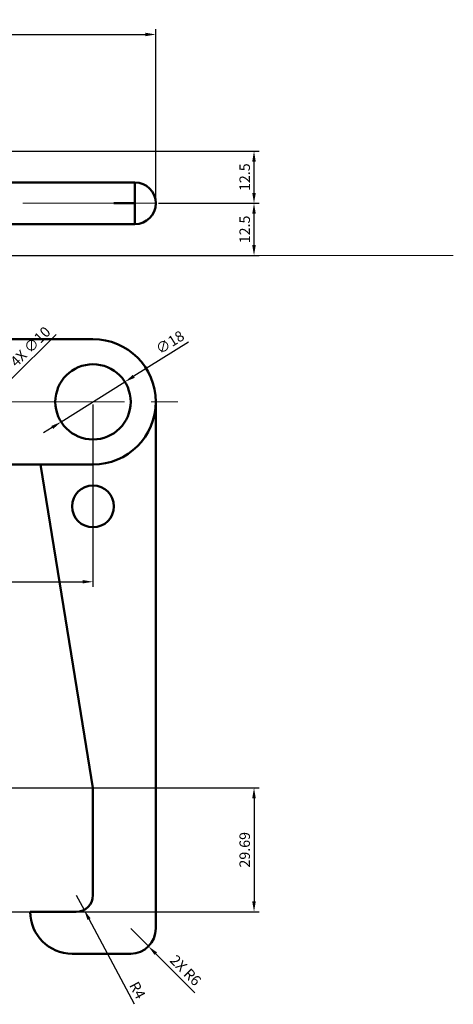
# Model space of a CAD drawing. Units: millimetres. Extents: x 5897 to 6166, y 4290 to 4529.
# Tile 2 of 2: x 6062 to 6166, y 4292 to 4528. Entities that reach past the tile are written whole.
import ezdxf

# ---------------------------------------------------------------- set-up
doc = ezdxf.new("R2010")
doc.units = ezdxf.units.MM
doc.linetypes.add('CENTER', pattern=[50.8, 31.75, -6.35, 6.35, -6.35])
for name, color, linetype, lineweight in [('M-CNTR', 1, 'CENTER', 18), ('M-CONS', 8, 'Continuous', 13), ('M-DIMS', 2, 'Continuous', 25), ('M-OUTL', 7, 'Continuous', 50)]:
    doc.layers.add(name, color=color, linetype=linetype, lineweight=lineweight)
doc.styles.get("Standard").update_dxf_attribs({"font": 'arial.ttf'})
doc.dimstyles.new('ISO-25', dxfattribs={"dimtxt": 2.5, "dimasz": 2.5, "dimexe": 1.25, "dimexo": 0.625, "dimtad": 1, "dimtxsty": 'Standard', "dimcen": 2.5, "dimadec": 0, "dimazin": 0, "dimtfac": 1, "dimtmove": 0, "dimatfit": 3, "dimfxl": 1, "dimarcsym": 0})

# ---------------------------------------------------------------- blocks, each defined once
blk = doc.blocks.new('*D9')
at = {"layer": 'Defpoints', "color": 0, "transparency": 16777216}
for p in [(5929.69, 4436.5), (6079.69, 4436.5), (6079.69, 4393.47)]:
    blk.add_point(p, dxfattribs=at)
at = {"layer": 'M-DIMS', "color": 0, "lineweight": -2, "transparency": 16777216}
for p, q in [((5929.69, 4435.88), (5929.69, 4392.22)), ((6079.69, 4435.88), (6079.69, 4392.22)), ((5932.19, 4393.47), (6077.19, 4393.47))]:
    blk.add_line(p, q, dxfattribs=at)
at = {"layer": 'M-DIMS', "color": 0, "transparency": 16777216}
for points in [[(5932.19, 4393.89), (5932.19, 4393.06), (5929.69, 4393.47)], [(6077.19, 4393.89), (6077.19, 4393.06), (6079.69, 4393.47)]]:
    blk.add_solid(points, dxfattribs=at)
at = {"layer": 'M-DIMS', "color": 0, "transparency": 16777216, "insert": (6004.69, 4395.37), "char_height": 2.5, "attachment_point": 5}
blk.add_mtext('150', dxfattribs=at)
blk = doc.blocks.new('*D10')
at = {"layer": 'Defpoints', "color": 0, "transparency": 16777216}
for p in [(6094.69, 4524.39), (5914.69, 4484), (6094.69, 4484)]:
    blk.add_point(p, dxfattribs=at)
at = {"layer": 'M-DIMS', "color": 0, "lineweight": -2, "transparency": 16777216}
for p, q in [((5914.69, 4484.63), (5914.69, 4525.64)), ((6094.69, 4484.63), (6094.69, 4525.64)), ((5917.19, 4524.39), (6092.19, 4524.39))]:
    blk.add_line(p, q, dxfattribs=at)
at = {"layer": 'M-DIMS', "color": 0, "transparency": 16777216}
for points in [[(5917.19, 4524.81), (5917.19, 4523.97), (5914.69, 4524.39)], [(6092.19, 4524.81), (6092.19, 4523.97), (6094.69, 4524.39)]]:
    blk.add_solid(points, dxfattribs=at)
at = {"layer": 'M-DIMS', "color": 0, "transparency": 16777216, "insert": (6004.69, 4526.29), "char_height": 2.5, "attachment_point": 5}
blk.add_mtext('180', dxfattribs=at)
blk = doc.blocks.new('*D14')
at = {"layer": 'Defpoints', "color": 0, "transparency": 16777216}
for p in [(6075.69, 4318.5), (6077.57, 4314.97)]:
    blk.add_point(p, dxfattribs=at)
at = {"layer": 'M-DIMS', "color": 0, "lineweight": -2, "transparency": 16777216}
for p, q in [((6075.69, 4318.5), (6077.57, 4314.97)), ((6089.62, 4292.39), (6078.75, 4312.77))]:
    blk.add_line(p, q, dxfattribs=at)
at = {"layer": 'M-DIMS', "color": 0, "transparency": 16777216}
blk.add_solid([(6079.11, 4312.96), (6078.38, 4312.57), (6077.57, 4314.97)], dxfattribs=at)
at = {"layer": 'M-DIMS', "color": 0, "transparency": 16777216, "insert": (6090.03, 4295.6), "char_height": 2.5, "attachment_point": 5, "rotation": 298.0738}
blk.add_mtext('R4', dxfattribs=at)
blk = doc.blocks.new('*D15')
at = {"layer": 'Defpoints', "color": 0, "transparency": 16777216}
for p in [(6087.31, 4441.29), (6072.07, 4431.72)]:
    blk.add_point(p, dxfattribs=at)
at = {"layer": 'M-DIMS', "color": 0, "lineweight": -2, "transparency": 16777216}
for p, q in [((6102.5, 4450.82), (6089.43, 4442.62)), ((6072.07, 4431.72), (6087.31, 4441.29)), ((6069.95, 4430.39), (6067.83, 4429.06))]:
    blk.add_line(p, q, dxfattribs=at)
at = {"layer": 'M-DIMS', "color": 0, "transparency": 16777216}
for points in [[(6089.21, 4442.97), (6089.65, 4442.26), (6087.31, 4441.29)], [(6069.73, 4430.74), (6070.17, 4430.03), (6072.07, 4431.72)]]:
    blk.add_solid(points, dxfattribs=at)
at = {"layer": 'M-DIMS', "color": 0, "transparency": 16777216, "insert": (6098.25, 4450.48), "char_height": 2.5, "attachment_point": 5, "rotation": 32.1239}
blk.add_mtext('∅18', dxfattribs=at)
blk = doc.blocks.new('*D20')
at = {"layer": 'Defpoints', "color": 0, "transparency": 16777216}
for p in [(6017.19, 4496.5), (6118.15, 4496.5), (6094.69, 4484)]:
    blk.add_point(p, dxfattribs=at)
at = {"layer": 'M-DIMS', "color": 0, "lineweight": -2, "transparency": 16777216}
for p, q in [((6017.81, 4496.5), (6119.4, 4496.5)), ((6118.15, 4486.5), (6118.15, 4494)), ((6095.31, 4484), (6119.4, 4484))]:
    blk.add_line(p, q, dxfattribs=at)
at = {"layer": 'M-DIMS', "color": 0, "transparency": 16777216}
for points in [[(6117.73, 4494), (6118.57, 4494), (6118.15, 4496.5)], [(6117.73, 4486.5), (6118.57, 4486.5), (6118.15, 4484)]]:
    blk.add_solid(points, dxfattribs=at)
at = {"layer": 'M-DIMS', "color": 0, "transparency": 16777216, "insert": (6116.25, 4490.25), "char_height": 2.5, "attachment_point": 5, "rotation": 90}
blk.add_mtext('12.5', dxfattribs=at)
blk = doc.blocks.new('*D21')
at = {"layer": 'Defpoints', "color": 0, "transparency": 16777216}
for p in [(6094.69, 4484), (6118.15, 4484), (6017.19, 4471.5)]:
    blk.add_point(p, dxfattribs=at)
at = {"layer": 'M-DIMS', "color": 0, "lineweight": -2, "transparency": 16777216}
for p, q in [((6095.31, 4484), (6119.4, 4484)), ((6118.15, 4474), (6118.15, 4481.5)), ((6017.81, 4471.5), (6119.4, 4471.5))]:
    blk.add_line(p, q, dxfattribs=at)
at = {"layer": 'M-DIMS', "color": 0, "transparency": 16777216}
for points in [[(6117.73, 4481.5), (6118.57, 4481.5), (6118.15, 4484)], [(6117.73, 4474), (6118.57, 4474), (6118.15, 4471.5)]]:
    blk.add_solid(points, dxfattribs=at)
at = {"layer": 'M-DIMS', "color": 0, "transparency": 16777216, "insert": (6116.25, 4477.75), "char_height": 2.5, "attachment_point": 5, "rotation": 90}
blk.add_mtext('12.5', dxfattribs=at)
blk = doc.blocks.new('*D25')
at = {"layer": 'Defpoints', "color": 0, "transparency": 16777216}
for p in [(5929.69, 4344.19), (5944.69, 4314.5), (6118.15, 4314.5)]:
    blk.add_point(p, dxfattribs=at)
at = {"layer": 'M-DIMS', "color": 0, "lineweight": -2, "transparency": 16777216}
for p, q in [((5930.31, 4344.19), (6119.4, 4344.19)), ((6118.15, 4341.69), (6118.15, 4317)), ((5945.31, 4314.5), (6119.4, 4314.5))]:
    blk.add_line(p, q, dxfattribs=at)
at = {"layer": 'M-DIMS', "color": 0, "transparency": 16777216}
for points in [[(6117.73, 4341.69), (6118.57, 4341.69), (6118.15, 4344.19)], [(6117.73, 4317), (6118.57, 4317), (6118.15, 4314.5)]]:
    blk.add_solid(points, dxfattribs=at)
at = {"layer": 'M-DIMS', "color": 0, "transparency": 16777216, "insert": (6116.25, 4329.35), "char_height": 2.5, "attachment_point": 5, "rotation": 90}
blk.add_mtext('29.69', dxfattribs=at)
blk = doc.blocks.new('*D35')
at = {"layer": 'Defpoints', "color": 0, "transparency": 16777216}
for p in [(6088.69, 4310.5), (6092.93, 4306.26)]:
    blk.add_point(p, dxfattribs=at)
at = {"layer": 'M-DIMS', "color": 0, "lineweight": -2, "transparency": 16777216}
for p, q in [((6088.69, 4310.5), (6092.93, 4306.26)), ((6104.03, 4295.16), (6094.7, 4304.49))]:
    blk.add_line(p, q, dxfattribs=at)
at = {"layer": 'M-DIMS', "color": 0, "transparency": 16777216}
blk.add_solid([(6094.99, 4304.79), (6094.4, 4304.2), (6092.93, 4306.26)], dxfattribs=at)
at = {"layer": 'M-DIMS', "color": 0, "transparency": 16777216, "insert": (6101.59, 4300.29), "char_height": 2.5, "attachment_point": 5, "rotation": 314.9957}
blk.add_mtext('2X R6', dxfattribs=at)
blk = doc.blocks.new('*D36')
at = {"layer": 'Defpoints', "color": 0, "transparency": 16777216}
for p in [(6058.23, 4440.03), (6051.14, 4432.97)]:
    blk.add_point(p, dxfattribs=at)
at = {"layer": 'M-DIMS', "color": 0, "lineweight": -2, "transparency": 16777216}
for p, q in [((6070.9, 4452.65), (6060, 4441.79)), ((6051.14, 4432.97), (6058.23, 4440.03)), ((6049.37, 4431.21), (6047.6, 4429.45))]:
    blk.add_line(p, q, dxfattribs=at)
at = {"layer": 'M-DIMS', "color": 0, "transparency": 16777216}
for points in [[(6059.71, 4442.09), (6060.3, 4441.5), (6058.23, 4440.03)], [(6049.08, 4431.5), (6049.67, 4430.91), (6051.14, 4432.97)]]:
    blk.add_solid(points, dxfattribs=at)
at = {"layer": 'M-DIMS', "color": 0, "transparency": 16777216, "insert": (6064.95, 4449.5), "char_height": 2.5, "attachment_point": 5, "rotation": 44.8833}
blk.add_mtext('4X ∅10', dxfattribs=at)

msp = doc.modelspace()

# ---------------------------------------------------------------- linework, layer by layer
at = {"layer": 'M-CNTR'}
for p, q in [((6094.688, 4484.002), (6004.688, 4484.002)), ((6004.688, 4436.502), (6105.301, 4436.502))]:
    msp.add_line(p, q, dxfattribs=at)
at = {"layer": 'M-CONS'}
for p, q in [((6165.744, 4471.502), (5997.188, 4471.502)), ((6004.688, 4471.502), (6165.744, 4471.502))]:
    msp.add_line(p, q, dxfattribs=at)
at = {"layer": 'M-OUTL'}
for p, q in [((6019.688, 4489.002), (6089.688, 4489.002)), ((6089.688, 4479.002), (6089.688, 4489.002)), ((6089.688, 4484.002), (6084.688, 4484.002)), ((6089.688, 4484.002), (6089.688, 4479.002)), ((6089.688, 4479.002), (6019.688, 4479.002)), ((6014.688, 4451.502), (6079.688, 4451.502)), ((6094.688, 4436.502), (6094.688, 4310.502)), ((6004.688, 4421.502), (6079.688, 4421.502)), ((6067.125, 4421.502), (6077.688, 4356.502)), ((6077.688, 4356.502), (6079.688, 4344.194)), ((6079.688, 4325.616), (6079.688, 4344.194)), ((6079.688, 4325.616), (6079.688, 4318.502)), ((6064.688, 4314.502), (6064.688, 4314.502)), ((6064.688, 4314.502), (6075.688, 4314.502)), ((6088.688, 4304.502), (6074.688, 4304.502)), ((6074.688, 4304.502), (6088.688, 4304.502)), ((6088.688, 4304.502), (6084.688, 4304.502))]:
    msp.add_line(p, q, dxfattribs=at)
for centre, radius in [((6079.688, 4436.502), 9), ((6079.688, 4411.502), 5)]:
    msp.add_circle(centre, radius, dxfattribs=at)
for centre, radius, start, end in [((6089.688, 4484.002), 5, 270, 90), ((6079.688, 4436.502), 15, 270, 90), ((6075.688, 4318.502), 4, 270, 360), ((6074.688, 4314.502), 10, 180, 270), ((6088.688, 4310.502), 6, 270, 0)]:
    msp.add_arc(centre, radius, start, end, dxfattribs=at)

# ---------------------------------------------------------------- dimensions: what is measured, and where the dimension line sits
at = {"layer": 'M-DIMS'}
for base, p1, p2, picture, middle in [((6094.688, 4524.388), (5914.688, 4484.002), (6094.688, 4484.002), '*D10', (6004.688, 4526.29)), ((6079.688, 4393.473), (5929.688, 4436.502), (6079.688, 4436.502), '*D9', (6004.688, 4395.374))]:
    dim = msp.add_linear_dim(base=base, p1=p1, p2=p2, dimstyle='ISO-25', override={"dimclrd": 0, "dimclre": 0, "dimclrt": 0}, dxfattribs=at)
    dim.commit()
    dim.dimension.update_dxf_attribs({"geometry": picture, "text_midpoint": middle})
for base, p1, p2, override, picture, middle in [((6118.151, 4496.502), (6094.688, 4484.002), (6017.188, 4496.502), {"dimdec": 1, "dimlfac": 1, "dimrnd": 0, "dimzin": 0, "dimdsep": 46, "dimlunit": 2}, '*D20', (6116.25, 4490.252)), ((6118.151, 4484.002), (6017.188, 4471.502), (6094.688, 4484.002), {"dimdec": 1, "dimlfac": 1, "dimrnd": 0, "dimzin": 0, "dimdsep": 46, "dimlunit": 2}, '*D21', (6116.25, 4477.752)), ((6118.151, 4314.502), (5929.688, 4344.194), (5944.688, 4314.502), {"dimdec": 2, "dimlfac": 1, "dimrnd": 0, "dimzin": 0, "dimdsep": 46, "dimlunit": 2}, '*D25', (6116.25, 4329.348))]:
    dim = msp.add_linear_dim(base=base, p1=p1, p2=p2, angle=90, dimstyle='ISO-25', override=override, dxfattribs=at)
    dim.commit()
    dim.dimension.update_dxf_attribs({"geometry": picture, "text_midpoint": middle})
dim = msp.add_diameter_dim_2p(p1=(6051.145, 4432.974), p2=(6058.23, 4440.03), text='4X <>', dimstyle='ISO-25', override={"dimdec": 0, "dimlfac": 1, "dimrnd": 0, "dimzin": 0, "dimdsep": 46, "dimlunit": 2}, dxfattribs=at)
dim.commit()
dim.dimension.update_dxf_attribs({"geometry": '*D36', "text_midpoint": (6066.337, 4448.104), "dimtype": 163})
dim = msp.add_diameter_dim_2p(p1=(6072.066, 4431.716), p2=(6087.31, 4441.288), dimstyle='ISO-25', override={"dimclrd": 0, "dimclre": 0, "dimclrt": 0}, dxfattribs=at)
dim.commit()
dim.dimension.update_dxf_attribs({"geometry": '*D15', "text_midpoint": (6099.297, 4448.814), "dimtype": 163})
dim = msp.add_radius_dim(center=(6075.688, 4318.502), mpoint=(6077.57, 4314.973), dimstyle='ISO-25', override={"dimclrd": 0, "dimclre": 0, "dimclrt": 0}, dxfattribs=at)
dim.commit()
dim.dimension.update_dxf_attribs({"geometry": '*D14', "text_midpoint": (6088.376, 4294.713), "dimtype": 164})
dim = msp.add_radius_dim(center=(6088.688, 4310.502), mpoint=(6092.93, 4306.259), text='2X <>', dimstyle='ISO-25', override={"dimdec": 0, "dimlfac": 1, "dimrnd": 0, "dimzin": 0, "dimdsep": 46, "dimlunit": 2}, dxfattribs=at)
dim.commit()
dim.dimension.update_dxf_attribs({"geometry": '*D35', "text_midpoint": (6101.591, 4300.286)})

doc.saveas('drawing.dxf')
